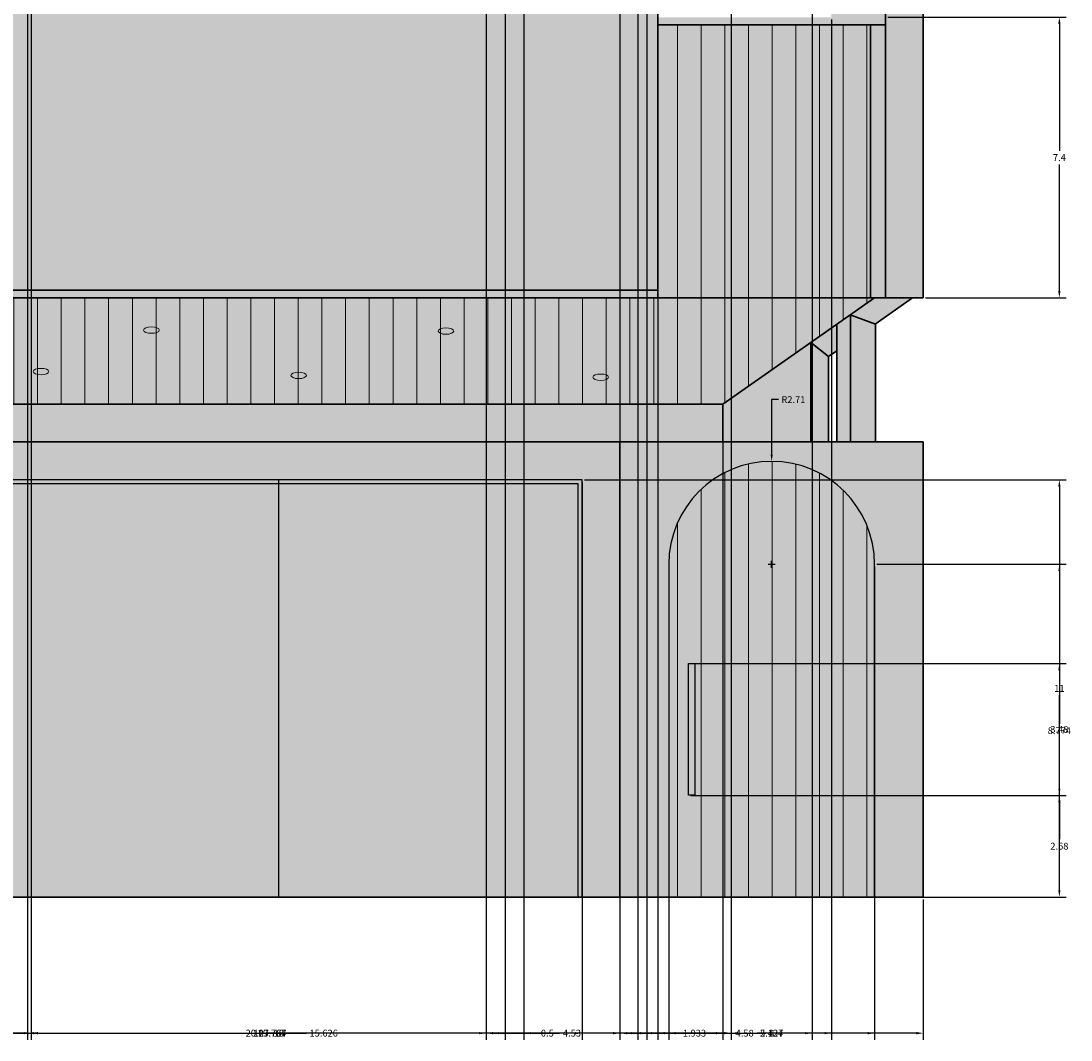
# Model space of a CAD drawing. Units: inches. Extents: x 18 to 59.8, y 2.7 to 81.2.
# Tile 2 of 9: x 32.1 to 59.8, y 2.7 to 29.5. Entities that reach past the tile are written whole.
import ezdxf

# ---------------------------------------------------------------- set-up
doc = ezdxf.new("R2010")
doc.units = ezdxf.units.IN
doc.header["$MEASUREMENT"] = 0
for name, color, linetype, lineweight in [('A-ANNO-DIMS', 2, 'Continuous', 18), ('A-DOOR', 3, 'Continuous', 25), ('A-ELEV', 7, 'Continuous', 35), ('A-ELEV-PATT', 8, 'Continuous', 13), ('E-LITE', 2, 'Continuous', 18)]:
    doc.layers.add(name, color=color, linetype=linetype, lineweight=lineweight)
doc.styles.get("Standard").update_dxf_attribs({"font": 'arial.ttf'})
doc.dimstyles.get("Standard").update_dxf_attribs({"dimtxt": 0.18, "dimasz": 0.18, "dimexe": 0.18, "dimexo": 0.0625, "dimgap": 0.09, "dimtad": 0, "dimtih": 1, "dimtoh": 1, "dimdec": 1, "dimzin": 0, "dimdsep": 46, "dimlunit": 3, "dimtxsty": 'Standard', "dimcen": 0.09, "dimadec": 0, "dimazin": 0, "dimtfac": 1, "dimtdec": 1, "dimtofl": 0, "dimtmove": 0, "dimatfit": 3, "dimfxl": 1, "dimtolj": 1, "dimtzin": 0, "dimarcsym": 0})

# ---------------------------------------------------------------- blocks, each defined once
blk = doc.blocks.new('LIGHT-SOFFIT-DOWN')
blk.add_ellipse((0.199, 0.085), major_axis=(0.207, 0), ratio=0.411448)
blk = doc.blocks.new('*D15')
at = {"layer": 'A-ANNO-DIMS', "color": 0, "lineweight": -2, "transparency": 16777216}
for p, q in [((54.922471, 29.640748), (59.629971, 29.640748)), ((59.449971, 29.460748), (59.449971, 26.120748)), ((59.449971, 22.420748), (59.449971, 25.760748)), ((55.922471, 22.240748), (59.629971, 22.240748))]:
    blk.add_line(p, q, dxfattribs=at)
at = {"layer": 'A-ANNO-DIMS', "color": 0, "transparency": 16777216}
for points in [[(59.419971, 29.460748), (59.479971, 29.460748), (59.449971, 29.640748)], [(59.419971, 22.420748), (59.479971, 22.420748), (59.449971, 22.240748)]]:
    blk.add_solid(points, dxfattribs=at)
at = {"layer": 'Defpoints', "color": 0, "transparency": 16777216}
for p in [(54.859971, 29.640748), (59.449971, 29.640748), (55.859971, 22.240748)]:
    blk.add_point(p, dxfattribs=at)
at = {"layer": 'A-ANNO-DIMS', "color": 0, "transparency": 16777216, "insert": (59.449971, 25.940748), "char_height": 0.18, "attachment_point": 5}
blk.add_mtext('\\A1;7.4', dxfattribs=at)
blk = doc.blocks.new('*D23')
at = {"layer": 'A-ANNO-DIMS', "color": 0, "lineweight": -2, "transparency": 16777216}
for p, q in [((48.86, 29.578), (48.86, 2.671)), ((53.44, 29.578), (53.44, 2.671)), ((49.04, 2.851), (50.822, 2.851)), ((53.26, 2.851), (51.478, 2.851))]:
    blk.add_line(p, q, dxfattribs=at)
at = {"layer": 'A-ANNO-DIMS', "color": 0, "transparency": 16777216}
for points in [[(49.04, 2.881), (49.04, 2.821), (48.86, 2.851)], [(53.26, 2.881), (53.26, 2.821), (53.44, 2.851)]]:
    blk.add_solid(points, dxfattribs=at)
at = {"layer": 'Defpoints', "color": 0, "transparency": 16777216}
for p in [(48.86, 29.641), (53.44, 29.641), (53.44, 2.851)]:
    blk.add_point(p, dxfattribs=at)
at = {"layer": 'A-ANNO-DIMS', "color": 0, "transparency": 16777216, "insert": (51.15, 2.851), "char_height": 0.18, "attachment_point": 5}
blk.add_mtext('\\A1;4.58', dxfattribs=at)
blk = doc.blocks.new('*D24')
at = {"layer": 'A-ANNO-DIMS', "color": 0, "lineweight": -2, "transparency": 16777216}
for p, q in [((48.86, 38.622), (48.86, 2.671)), ((50.793, 38.622), (50.793, 2.671)), ((49.04, 2.851), (49.441, 2.851)), ((50.613, 2.851), (50.212, 2.851))]:
    blk.add_line(p, q, dxfattribs=at)
at = {"layer": 'A-ANNO-DIMS', "color": 0, "transparency": 16777216}
for points in [[(49.04, 2.881), (49.04, 2.821), (48.86, 2.851)], [(50.613, 2.881), (50.613, 2.821), (50.793, 2.851)]]:
    blk.add_solid(points, dxfattribs=at)
at = {"layer": 'Defpoints', "color": 0, "transparency": 16777216}
for p in [(48.86, 38.685), (50.793, 38.685), (50.793, 2.851)]:
    blk.add_point(p, dxfattribs=at)
at = {"layer": 'A-ANNO-DIMS', "color": 0, "transparency": 16777216, "insert": (49.826, 2.851), "char_height": 0.18, "attachment_point": 5}
blk.add_mtext('\\A1;1.933', dxfattribs=at)
blk = doc.blocks.new('*D25')
at = {"layer": 'A-ANNO-DIMS', "color": 0, "lineweight": -2, "transparency": 16777216}
for p, q in [((50.793, 41.253), (50.793, 2.671)), ((52.927, 41.253), (52.927, 2.671)), ((50.973, 2.851), (51.465, 2.851)), ((52.747, 2.851), (52.255, 2.851))]:
    blk.add_line(p, q, dxfattribs=at)
at = {"layer": 'A-ANNO-DIMS', "color": 0, "transparency": 16777216}
for points in [[(50.973, 2.881), (50.973, 2.821), (50.793, 2.851)], [(52.747, 2.881), (52.747, 2.821), (52.927, 2.851)]]:
    blk.add_solid(points, dxfattribs=at)
at = {"layer": 'Defpoints', "color": 0, "transparency": 16777216}
for p in [(50.793, 41.316), (52.927, 41.316), (52.927, 2.851)]:
    blk.add_point(p, dxfattribs=at)
at = {"layer": 'A-ANNO-DIMS', "color": 0, "transparency": 16777216, "insert": (51.86, 2.851), "char_height": 0.18, "attachment_point": 5}
blk.add_mtext('\\A1;2.134', dxfattribs=at)
blk = doc.blocks.new('*D29')
at = {"layer": 'A-ANNO-DIMS', "color": 0, "lineweight": -2, "transparency": 16777216}
for p, q in [((29.86, 6.378), (29.86, 2.671)), ((47.86, 6.378), (47.86, 2.671)), ((30.04, 2.851), (38.649, 2.851)), ((47.68, 2.851), (39.071, 2.851))]:
    blk.add_line(p, q, dxfattribs=at)
at = {"layer": 'A-ANNO-DIMS', "color": 0, "transparency": 16777216}
for points in [[(30.04, 2.881), (30.04, 2.821), (29.86, 2.851)], [(47.68, 2.881), (47.68, 2.821), (47.86, 2.851)]]:
    blk.add_solid(points, dxfattribs=at)
at = {"layer": 'Defpoints', "color": 0, "transparency": 16777216}
for p in [(29.86, 6.441), (47.86, 6.441), (47.86, 2.851)]:
    blk.add_point(p, dxfattribs=at)
at = {"layer": 'A-ANNO-DIMS', "color": 0, "transparency": 16777216, "insert": (38.86, 2.851), "char_height": 0.18, "attachment_point": 5}
blk.add_mtext('\\A1;18', dxfattribs=at)
blk = doc.blocks.new('*D30')
at = {"layer": 'A-ANNO-DIMS', "color": 0, "lineweight": -2, "transparency": 16777216}
for p, q in [((47.86, 6.378), (47.86, 2.671)), ((55.86, 6.378), (55.86, 2.671)), ((48.04, 2.851), (51.711, 2.851)), ((55.68, 2.851), (52.009, 2.851))]:
    blk.add_line(p, q, dxfattribs=at)
at = {"layer": 'A-ANNO-DIMS', "color": 0, "transparency": 16777216}
for points in [[(48.04, 2.881), (48.04, 2.821), (47.86, 2.851)], [(55.68, 2.881), (55.68, 2.821), (55.86, 2.851)]]:
    blk.add_solid(points, dxfattribs=at)
at = {"layer": 'Defpoints', "color": 0, "transparency": 16777216}
for p in [(47.86, 6.441), (55.86, 6.441), (55.86, 2.851)]:
    blk.add_point(p, dxfattribs=at)
at = {"layer": 'A-ANNO-DIMS', "color": 0, "transparency": 16777216, "insert": (51.86, 2.851), "char_height": 0.18, "attachment_point": 5}
blk.add_mtext('\\A1;8', dxfattribs=at)
blk = doc.blocks.new('*D33')
at = {"layer": 'A-ANNO-DIMS', "color": 0, "lineweight": -2, "transparency": 16777216}
for p, q in [((49.148, 15.152), (49.148, 2.671)), ((54.576, 15.152), (54.576, 2.671)), ((49.328, 2.851), (51.468, 2.851)), ((54.396, 2.851), (52.256, 2.851))]:
    blk.add_line(p, q, dxfattribs=at)
at = {"layer": 'A-ANNO-DIMS', "color": 0, "transparency": 16777216}
for points in [[(49.328, 2.881), (49.328, 2.821), (49.148, 2.851)], [(54.396, 2.881), (54.396, 2.821), (54.576, 2.851)]]:
    blk.add_solid(points, dxfattribs=at)
at = {"layer": 'Defpoints', "color": 0, "transparency": 16777216}
for p in [(49.148, 15.215), (54.576, 15.215), (54.576, 2.851)]:
    blk.add_point(p, dxfattribs=at)
at = {"layer": 'A-ANNO-DIMS', "color": 0, "transparency": 16777216, "insert": (51.862, 2.851), "char_height": 0.18, "attachment_point": 5}
blk.add_mtext('\\A1;5.427', dxfattribs=at)
blk = doc.blocks.new('*D34')
at = {"layer": 'A-ANNO-DIMS', "color": 0, "lineweight": -2, "transparency": 16777216}
for p, q in [((30.86, 17.378), (30.86, 2.671)), ((46.86, 17.378), (46.86, 2.671)), ((31.04, 2.851), (38.65, 2.851)), ((46.68, 2.851), (39.07, 2.851))]:
    blk.add_line(p, q, dxfattribs=at)
at = {"layer": 'A-ANNO-DIMS', "color": 0, "transparency": 16777216}
for points in [[(31.04, 2.881), (31.04, 2.821), (30.86, 2.851)], [(46.68, 2.881), (46.68, 2.821), (46.86, 2.851)]]:
    blk.add_solid(points, dxfattribs=at)
at = {"layer": 'Defpoints', "color": 0, "transparency": 16777216}
for p in [(30.86, 17.441), (46.86, 17.441), (46.86, 2.851)]:
    blk.add_point(p, dxfattribs=at)
at = {"layer": 'A-ANNO-DIMS', "color": 0, "transparency": 16777216, "insert": (38.86, 2.851), "char_height": 0.18, "attachment_point": 5}
blk.add_mtext('\\A1;16', dxfattribs=at)
blk = doc.blocks.new('*D41')
at = {"layer": 'A-ANNO-DIMS', "color": 0, "lineweight": -2, "transparency": 16777216}
for p, q in [((54.638, 15.215), (59.63, 15.215)), ((59.45, 15.035), (59.45, 11.01)), ((59.45, 6.621), (59.45, 10.646)), ((54.638, 6.441), (59.63, 6.441))]:
    blk.add_line(p, q, dxfattribs=at)
at = {"layer": 'A-ANNO-DIMS', "color": 0, "transparency": 16777216}
for points in [[(59.42, 15.035), (59.48, 15.035), (59.45, 15.215)], [(59.42, 6.621), (59.48, 6.621), (59.45, 6.441)]]:
    blk.add_solid(points, dxfattribs=at)
at = {"layer": 'Defpoints', "color": 0, "transparency": 16777216}
for p in [(54.576, 15.215), (59.45, 15.215), (54.576, 6.441)]:
    blk.add_point(p, dxfattribs=at)
at = {"layer": 'A-ANNO-DIMS', "color": 0, "transparency": 16777216, "insert": (59.45, 10.828), "char_height": 0.18, "attachment_point": 5}
blk.add_mtext('\\A1;8.774', dxfattribs=at)
blk = doc.blocks.new('*D42')
at = {"layer": 'A-ANNO-DIMS', "color": 0, "lineweight": -2, "transparency": 16777216}
for p, q in [((46.922, 17.441), (59.63, 17.441)), ((59.45, 17.261), (59.45, 12.121)), ((59.45, 6.621), (59.45, 11.76)), ((46.922, 6.441), (59.63, 6.441))]:
    blk.add_line(p, q, dxfattribs=at)
at = {"layer": 'A-ANNO-DIMS', "color": 0, "transparency": 16777216}
for points in [[(59.42, 17.261), (59.48, 17.261), (59.45, 17.441)], [(59.42, 6.621), (59.48, 6.621), (59.45, 6.441)]]:
    blk.add_solid(points, dxfattribs=at)
at = {"layer": 'Defpoints', "color": 0, "transparency": 16777216}
for p in [(46.86, 17.441), (59.45, 17.441), (46.86, 6.441)]:
    blk.add_point(p, dxfattribs=at)
at = {"layer": 'A-ANNO-DIMS', "color": 0, "transparency": 16777216, "insert": (59.45, 11.941), "char_height": 0.18, "attachment_point": 5}
blk.add_mtext('\\A1;11', dxfattribs=at)
blk = doc.blocks.new('*D43')
at = {"layer": 'A-ANNO-DIMS', "color": 0, "lineweight": -2, "transparency": 16777216}
for p, q in [((49.728, 12.602), (59.63, 12.602)), ((59.45, 12.422), (59.45, 11.044)), ((59.45, 9.302), (59.45, 10.68)), ((49.728, 9.122), (59.63, 9.122))]:
    blk.add_line(p, q, dxfattribs=at)
at = {"layer": 'A-ANNO-DIMS', "color": 0, "transparency": 16777216}
for points in [[(59.42, 12.422), (59.48, 12.422), (59.45, 12.602)], [(59.42, 9.302), (59.48, 9.302), (59.45, 9.122)]]:
    blk.add_solid(points, dxfattribs=at)
at = {"layer": 'Defpoints', "color": 0, "transparency": 16777216}
for p in [(49.666, 12.602), (59.45, 12.602), (49.666, 9.122)]:
    blk.add_point(p, dxfattribs=at)
at = {"layer": 'A-ANNO-DIMS', "color": 0, "transparency": 16777216, "insert": (59.45, 10.862), "char_height": 0.18, "attachment_point": 5}
blk.add_mtext('\\A1;3.48', dxfattribs=at)
blk = doc.blocks.new('*D44')
at = {"layer": 'A-ANNO-DIMS', "color": 0, "lineweight": -2, "transparency": 16777216}
for p, q in [((49.728, 9.122), (59.63, 9.122)), ((59.45, 8.942), (59.45, 7.964)), ((59.45, 6.621), (59.45, 7.6)), ((49.211, 6.441), (59.63, 6.441))]:
    blk.add_line(p, q, dxfattribs=at)
at = {"layer": 'A-ANNO-DIMS', "color": 0, "transparency": 16777216}
for points in [[(59.42, 8.942), (59.48, 8.942), (59.45, 9.122)], [(59.42, 6.621), (59.48, 6.621), (59.45, 6.441)]]:
    blk.add_solid(points, dxfattribs=at)
at = {"layer": 'Defpoints', "color": 0, "transparency": 16777216}
for p in [(49.666, 9.122), (59.45, 9.122), (49.148, 6.441)]:
    blk.add_point(p, dxfattribs=at)
at = {"layer": 'A-ANNO-DIMS', "color": 0, "transparency": 16777216, "insert": (59.45, 7.782), "char_height": 0.18, "attachment_point": 5}
blk.add_mtext('\\A1;2.68', dxfattribs=at)
blk = doc.blocks.new('*D46')
at = {"layer": 'A-ANNO-DIMS', "color": 0, "lineweight": -2, "transparency": 16777216}
for p, q in [((26.811, 19.378), (26.811, 2.671)), ((50.578, 19.378), (50.578, 2.671)), ((26.991, 2.851), (38.229, 2.851)), ((50.398, 2.851), (39.159, 2.851))]:
    blk.add_line(p, q, dxfattribs=at)
at = {"layer": 'A-ANNO-DIMS', "color": 0, "transparency": 16777216}
for points in [[(26.991, 2.881), (26.991, 2.821), (26.811, 2.851)], [(50.398, 2.881), (50.398, 2.821), (50.578, 2.851)]]:
    blk.add_solid(points, dxfattribs=at)
at = {"layer": 'Defpoints', "color": 0, "transparency": 16777216}
for p in [(26.811, 19.441), (50.578, 19.441), (50.578, 2.851)]:
    blk.add_point(p, dxfattribs=at)
at = {"layer": 'A-ANNO-DIMS', "color": 0, "transparency": 16777216, "insert": (38.694, 2.851), "char_height": 0.18, "attachment_point": 5}
blk.add_mtext('\\A1;23.767', dxfattribs=at)
blk = doc.blocks.new('*D54')
at = {"layer": 'A-ANNO-DIMS', "color": 0, "lineweight": -2, "transparency": 16777216}
for p, q in [((28.258, 33.771), (28.258, 2.671)), ((48.33, 33.352), (48.33, 2.671)), ((28.438, 2.851), (37.899, 2.851)), ((48.15, 2.851), (38.689, 2.851))]:
    blk.add_line(p, q, dxfattribs=at)
at = {"layer": 'A-ANNO-DIMS', "color": 0, "transparency": 16777216}
for points in [[(28.438, 2.881), (28.438, 2.821), (28.258, 2.851)], [(48.15, 2.881), (48.15, 2.821), (48.33, 2.851)]]:
    blk.add_solid(points, dxfattribs=at)
at = {"layer": 'Defpoints', "color": 0, "transparency": 16777216}
for p in [(28.258, 33.834), (48.33, 33.414), (48.33, 2.851)]:
    blk.add_point(p, dxfattribs=at)
at = {"layer": 'A-ANNO-DIMS', "color": 0, "transparency": 16777216, "insert": (38.294, 2.851), "char_height": 0.18, "attachment_point": 5}
blk.add_mtext('\\A1;20.07', dxfattribs=at)
blk = doc.blocks.new('*D55')
at = {"layer": 'A-ANNO-DIMS', "color": 0, "lineweight": -2, "transparency": 16777216}
for p, q in [((44.83, 33.671), (44.83, 2.671)), ((45.33, 33.671), (45.33, 2.671)), ((44.65, 2.851), (44.47, 2.851)), ((45.51, 2.851), (45.69, 2.851))]:
    blk.add_line(p, q, dxfattribs=at)
at = {"layer": 'A-ANNO-DIMS', "color": 0, "transparency": 16777216}
for points in [[(44.65, 2.881), (44.65, 2.821), (44.83, 2.851)], [(45.51, 2.881), (45.51, 2.821), (45.33, 2.851)]]:
    blk.add_solid(points, dxfattribs=at)
at = {"layer": 'Defpoints', "color": 0, "transparency": 16777216}
for p in [(44.83, 33.734), (45.33, 33.734), (45.33, 2.851)]:
    blk.add_point(p, dxfattribs=at)
at = {"layer": 'A-ANNO-DIMS', "color": 0, "transparency": 16777216, "insert": (45.945, 2.851), "char_height": 0.18, "attachment_point": 5}
blk.add_mtext('\\A1;0.5', dxfattribs=at)
blk = doc.blocks.new('*D56')
at = {"layer": 'A-ANNO-DIMS', "color": 0, "lineweight": -2, "transparency": 16777216}
for p, q in [((30.406, 31.378), (30.406, 2.671)), ((32.33, 31.378), (32.33, 2.671)), ((30.586, 2.851), (30.983, 2.851)), ((32.15, 2.851), (31.753, 2.851))]:
    blk.add_line(p, q, dxfattribs=at)
at = {"layer": 'A-ANNO-DIMS', "color": 0, "transparency": 16777216}
for points in [[(30.586, 2.881), (30.586, 2.821), (30.406, 2.851)], [(32.15, 2.881), (32.15, 2.821), (32.33, 2.851)]]:
    blk.add_solid(points, dxfattribs=at)
at = {"layer": 'Defpoints', "color": 0, "transparency": 16777216}
for p in [(30.406, 31.441), (32.33, 31.441), (32.33, 2.851)]:
    blk.add_point(p, dxfattribs=at)
at = {"layer": 'A-ANNO-DIMS', "color": 0, "transparency": 16777216, "insert": (31.368, 2.851), "char_height": 0.18, "attachment_point": 5}
blk.add_mtext('\\A1;1.924', dxfattribs=at)
blk = doc.blocks.new('*D57')
at = {"layer": 'A-ANNO-DIMS', "color": 0, "lineweight": -2, "transparency": 16777216}
for p, q in [((32.33, 31.378), (32.33, 2.671)), ((44.33, 31.378), (44.33, 2.671)), ((32.51, 2.851), (38.121, 2.851)), ((44.15, 2.851), (38.54, 2.851))]:
    blk.add_line(p, q, dxfattribs=at)
at = {"layer": 'A-ANNO-DIMS', "color": 0, "transparency": 16777216}
for points in [[(32.51, 2.881), (32.51, 2.821), (32.33, 2.851)], [(44.15, 2.881), (44.15, 2.821), (44.33, 2.851)]]:
    blk.add_solid(points, dxfattribs=at)
at = {"layer": 'Defpoints', "color": 0, "transparency": 16777216}
for p in [(32.33, 31.441), (44.33, 31.441), (44.33, 2.851)]:
    blk.add_point(p, dxfattribs=at)
at = {"layer": 'A-ANNO-DIMS', "color": 0, "transparency": 16777216, "insert": (38.33, 2.851), "char_height": 0.18, "attachment_point": 5}
blk.add_mtext('\\A1;12', dxfattribs=at)
blk = doc.blocks.new('*D58')
at = {"layer": 'A-ANNO-DIMS', "color": 0, "lineweight": -2, "transparency": 16777216}
for p, q in [((48.86, 38.622), (48.86, 2.671)), ((44.33, 31.378), (44.33, 2.671)), ((44.51, 2.851), (46.268, 2.851)), ((48.68, 2.851), (46.923, 2.851))]:
    blk.add_line(p, q, dxfattribs=at)
at = {"layer": 'A-ANNO-DIMS', "color": 0, "transparency": 16777216}
for points in [[(44.51, 2.881), (44.51, 2.821), (44.33, 2.851)], [(48.68, 2.881), (48.68, 2.821), (48.86, 2.851)]]:
    blk.add_solid(points, dxfattribs=at)
at = {"layer": 'Defpoints', "color": 0, "transparency": 16777216}
for p in [(48.86, 38.685), (44.33, 31.441), (48.86, 2.851)]:
    blk.add_point(p, dxfattribs=at)
at = {"layer": 'A-ANNO-DIMS', "color": 0, "transparency": 16777216, "insert": (46.595, 2.851), "char_height": 0.18, "attachment_point": 5}
blk.add_mtext('\\A1;4.53', dxfattribs=at)
blk = doc.blocks.new('*D61')
at = {"layer": 'A-ANNO-DIMS', "color": 0, "lineweight": -2, "transparency": 16777216}
for p, q in [((32.234, 49.378), (32.234, 2.671)), ((47.86, 49.378), (47.86, 2.671)), ((32.414, 2.851), (39.592, 2.851)), ((47.68, 2.851), (40.502, 2.851))]:
    blk.add_line(p, q, dxfattribs=at)
at = {"layer": 'A-ANNO-DIMS', "color": 0, "transparency": 16777216}
for points in [[(32.414, 2.881), (32.414, 2.821), (32.234, 2.851)], [(47.68, 2.881), (47.68, 2.821), (47.86, 2.851)]]:
    blk.add_solid(points, dxfattribs=at)
at = {"layer": 'Defpoints', "color": 0, "transparency": 16777216}
for p in [(32.234, 49.441), (47.86, 49.441), (47.86, 2.851)]:
    blk.add_point(p, dxfattribs=at)
at = {"layer": 'A-ANNO-DIMS', "color": 0, "transparency": 16777216, "insert": (40.047, 2.851), "char_height": 0.18, "attachment_point": 5}
blk.add_mtext('\\A1;15.626', dxfattribs=at)
blk = doc.blocks.new('*D66')
at = {"layer": 'A-ANNO-DIMS', "color": 0, "lineweight": -2, "transparency": 16777216}
for p, q in [((28.804, 51.378), (28.804, 2.671)), ((48.567, 51.179), (48.567, 2.671)), ((28.984, 2.851), (38.231, 2.851)), ((48.387, 2.851), (39.14, 2.851))]:
    blk.add_line(p, q, dxfattribs=at)
at = {"layer": 'A-ANNO-DIMS', "color": 0, "transparency": 16777216}
for points in [[(28.984, 2.881), (28.984, 2.821), (28.804, 2.851)], [(48.387, 2.881), (48.387, 2.821), (48.567, 2.851)]]:
    blk.add_solid(points, dxfattribs=at)
at = {"layer": 'Defpoints', "color": 0, "transparency": 16777216}
for p in [(28.804, 51.441), (48.567, 51.242), (48.567, 2.851)]:
    blk.add_point(p, dxfattribs=at)
at = {"layer": 'A-ANNO-DIMS', "color": 0, "transparency": 16777216, "insert": (38.685, 2.851), "char_height": 0.18, "attachment_point": 5}
blk.add_mtext('\\A1;19.764', dxfattribs=at)
blk = doc.blocks.new('*D68')
at = {"layer": 'A-ANNO-DIMS', "color": 0, "lineweight": -2, "transparency": 16777216}
for p, q in [((52.042, 19.557), (51.862, 19.557)), ((51.862, 19.557), (51.862, 18.109)), ((51.862, 15.125), (51.862, 15.305)), ((51.772, 15.215), (51.952, 15.215))]:
    blk.add_line(p, q, dxfattribs=at)
at = {"layer": 'A-ANNO-DIMS', "color": 0, "transparency": 16777216}
blk.add_solid([(51.832, 18.109), (51.892, 18.109), (51.862, 17.929)], dxfattribs=at)
at = {"layer": 'Defpoints', "color": 0, "transparency": 16777216}
for p in [(51.862, 17.929), (51.862, 15.215)]:
    blk.add_point(p, dxfattribs=at)
at = {"layer": 'A-ANNO-DIMS', "color": 0, "transparency": 16777216, "insert": (52.435, 19.557), "char_height": 0.18, "attachment_point": 5}
blk.add_mtext('\\A1;R2.71', dxfattribs=at)

msp = doc.modelspace()

# ---------------------------------------------------------------- hatches: boundary and pattern name
at = {"layer": 'A-ELEV-PATT'}
h = msp.add_hatch(color=256, dxfattribs=at)
h.set_gradient(color1=(255, 255, 255), color2=(199, 200, 202))
h.paths.add_polyline_path([(38.86, 75.4521, 0.4125527), (36.86, 77.4407), (21.86, 77.4407), (21.86, 22.4407), (22.86, 22.4407), (48.86, 22.4407), (48.86, 30.9234, 0.4074473), (48.3302, 31.4407), (30.4061, 31.4407, -0.7603989), (34.0116, 44.4407), (47.86, 44.4407, -0.4142136), (48.86, 43.4407), (48.86, 48.4407, 0.4142136), (47.86, 49.4407), (32.2338, 49.4407, -0.2243142), (27.8411, 52.8427, -0.8480129), (38.86, 61.4407)])
h.paths.add_polyline_path([(55.86, 77.4407), (54.86, 77.4407), (54.86, 22.2407), (55.86, 22.2407)])
h.paths.add_polyline_path([(54.86, 51.5407), (53.4401, 51.5407), (53.4401, 29.6407), (54.86, 29.6407)])
h.paths.add_polyline_path([(54.86, 61.4407), (53.4401, 57.4407), (53.4401, 51.6407), (54.86, 51.6407)])
h.paths.add_polyline_path([(54.86, 29.4407), (54.471, 29.4407), (54.471, 22.2407), (54.86, 22.2407)])
h.paths.add_polyline_path([(55.5745, 22.2407), (54.86, 22.2407), (54.5745, 22.2407), (53.9347, 21.7925), (54.5877, 21.5495)])
h.paths.add_polyline_path([(54.5991, 21.5452), (53.9443, 21.789), (53.9443, 18.4407), (54.5991, 18.4407)])
h.paths.add_polyline_path([(53.9443, 21.789), (53.9347, 21.7925), (53.5816, 21.5452), (53.5816, 18.4407), (53.9443, 18.4407)])
h.paths.add_polyline_path([(53.3648, 20.6928), (52.8956, 21.0646), (52.8956, 18.4407), (53.3648, 18.4407)])
h.paths.add_polyline_path([(52.8956, 21.0646), (50.5775, 19.4407), (50.5775, 18.4407), (52.8956, 18.4407)])
h.paths.add_polyline_path([(53.5816, 21.5452), (52.8956, 21.0646), (53.3648, 20.6928), (53.5816, 20.8447)])
h.paths.add_polyline_path([(26.8109, 19.4407), (24.9672, 20.8407), (24.9672, 18.4407), (26.8109, 18.4407)])
h.paths.add_polyline_path([(24.9672, 20.8407), (24.4165, 20.8427), (24.4165, 18.4407), (24.9672, 18.4407)])
h.paths.add_polyline_path([(24.4165, 20.8427), (24.4165, 21.2589), (24.0588, 21.5305), (24.0301, 21.5183), (24.0301, 18.4407), (24.4165, 18.4407)])
h.paths.add_polyline_path([(24.0301, 21.5183), (23.4165, 21.2589), (23.4165, 18.4407), (24.0301, 18.4407)])
h.paths.add_polyline_path([(24.0301, 21.5183), (24.0588, 21.5305), (23.1234, 22.2407), (22.1234, 22.2407), (23.4165, 21.2589)])
h.paths.add_polyline_path([(24.4165, 21.2589), (24.4165, 20.8427), (24.9672, 20.8407)])
h.paths.add_polyline_path([(47.86, 18.4407), (29.86, 18.4407), (29.86, 6.4407), (30.86, 6.4407), (30.86, 17.4407), (38.86, 17.4407), (46.86, 17.4407), (46.86, 6.4407), (47.86, 6.4407)])
h.paths.add_polyline_path([(54.5756, 15.215), (54.5756, 6.4407), (55.86, 6.4407), (55.86, 18.4407), (47.86, 18.4407), (47.86, 6.4407), (49.1482, 6.4407), (49.1482, 15.215, -1)])
h = msp.add_hatch(color=256, dxfattribs=at)
h.paths.add_polyline_path([(27.8411, 52.8427, -0.7443789), (36.86, 61.4407), (38.86, 61.4407, 0.8480129)])
h.paths.add_polyline_path([(47.86, 44.4407), (34.0116, 44.4407, 0.7603989), (30.4061, 31.4407, -0.7376246), (34.0116, 43.4407), (47.86, 43.4407, -0.4142136), (48.86, 42.4407), (48.86, 43.4407, 0.4142136)])
h.paths.add_polyline_path([(54.5756, 15.215), (54.5756, 6.4407), (55.86, 6.4407), (55.86, 18.4407), (47.86, 18.4407), (47.86, 6.4407), (49.1482, 6.4407), (49.1482, 15.215, -1)])
h.paths.add_polyline_path([(47.86, 18.4407), (29.86, 18.4407), (29.86, 6.4407), (30.86, 6.4407), (30.86, 17.4407), (38.86, 17.4407), (46.86, 17.4407), (46.86, 6.4407), (47.86, 6.4407)])
h.paths.add_polyline_path([(55.86, 77.4407), (54.86, 77.4407), (54.86, 22.2407), (55.86, 22.2407)])
h = msp.add_hatch(color=256, dxfattribs=at)
h.dxf.hatch_style = 1
h.paths.add_polyline_path([(54.86, 69.4407), (38.86, 69.4407), (38.86, 61.4407), (54.86, 61.4407)])
h.paths.add_polyline_path([(54.86, 61.4407), (38.86, 61.4407), (36.86, 61.4407, 0.443414), (27.6986, 58.4407), (48.86, 58.4407), (48.86, 57.4407), (53.4401, 57.4407)])
h.paths.add_polyline_path([(37.4994, 59.9399), (37.4994, 59.8198, -2.4106499), (37.1187, 59.8198), (37.1187, 59.9399)], flags=16)
h.paths.add_polyline_path([(42.6125, 59.8012), (42.6125, 59.9213), (42.9933, 59.9213), (42.9933, 59.8012, -2.4106499)], flags=16)
h.paths.add_polyline_path([(49.5965, 59.971), (49.5965, 60.091), (49.9773, 60.091), (49.9773, 59.971, -2.4106499)], flags=16)
h.paths.add_polyline_path([(44.4671, 57.0407), (32.6671, 57.0407), (32.6671, 56.0407), (44.4671, 56.0407)])
h.paths.add_polyline_path([(47.86, 43.4407), (46.86, 43.4407), (34.0116, 43.4407, 0.2012983), (29.3481, 41.4407), (47.86, 41.4407, 1)])
h.paths.add_polyline_path([(36.5542, 42.5145), (36.5542, 42.6346), (36.9349, 42.6346), (36.9349, 42.5145, -2.4106499)], flags=16)
h.paths.add_polyline_path([(42.939, 42.5402), (42.939, 42.6603), (43.3198, 42.6603), (43.3198, 42.5402, -2.4106499)], flags=16)
h.paths.add_polyline_path([(54.471, 29.4407), (48.86, 29.4407), (48.86, 22.2407), (54.471, 22.2407)])
h.paths.add_polyline_path([(54.5745, 22.2407), (23.1234, 22.2407), (26.8109, 19.4407), (50.5775, 19.4407)])
h.paths.add_polyline_path([(54.5756, 15.215, 1), (49.1482, 15.215), (49.1482, 6.4407), (54.5756, 6.4407)])
h.paths.add_polyline_path([(49.8323, 12.602), (49.8323, 9.1225), (49.6657, 9.1225), (49.6657, 12.602)], flags=16)
h = msp.add_hatch(dxfattribs=at)
h.set_pattern_fill('ANSI31', color=256, scale=5, angle=45, style=0)
h.paths.add_polyline_path([(54.86, 69.4407), (38.86, 69.4407), (38.86, 61.4407), (54.86, 61.4407)])
h.paths.add_polyline_path([(54.86, 61.4407), (38.86, 61.4407), (36.86, 61.4407, 0.443414), (27.6986, 58.4407), (48.86, 58.4407), (48.86, 57.4407), (53.4401, 57.4407)])
h.paths.add_polyline_path([(37.1661, 59.8577), (37.1187, 59.8577), (37.1187, 59.9399), (37.4994, 59.9399), (37.4994, 59.8577), (37.452, 59.8577, -3.476462)], flags=16)
h.paths.add_polyline_path([(42.66, 59.8391), (42.6125, 59.8391), (42.6125, 59.9213), (42.9933, 59.9213), (42.9933, 59.8391), (42.9458, 59.8391, -3.476462)], flags=16)
h.paths.add_polyline_path([(49.644, 60.0088), (49.5965, 60.0088), (49.5965, 60.091), (49.9773, 60.091), (49.9773, 60.0088), (49.9298, 60.0088, -3.476462)], flags=16)
h.paths.add_polyline_path([(44.4671, 57.0407), (32.6671, 57.0407), (32.6671, 56.0407), (44.4671, 56.0407)])
h.paths.add_polyline_path([(47.86, 43.4407), (46.86, 43.4407), (34.0116, 43.4407, 0.2012983), (29.3481, 41.4407), (47.86, 41.4407, 1)])
h.paths.add_polyline_path([(36.6016, 42.5524), (36.5542, 42.5524), (36.5542, 42.6346), (36.9349, 42.6346), (36.9349, 42.5524), (36.8875, 42.5524, -3.476462)], flags=16)
h.paths.add_polyline_path([(42.9865, 42.578), (42.939, 42.578), (42.939, 42.6603), (43.3198, 42.6603), (43.3198, 42.578), (43.2723, 42.578, -3.476462)], flags=16)
h.paths.add_polyline_path([(54.471, 29.4407), (48.86, 29.4407), (48.86, 22.2407), (54.471, 22.2407)])
h.paths.add_polyline_path([(54.5745, 22.2407), (23.1234, 22.2407), (26.8109, 19.4407), (50.5775, 19.4407)])
h.paths.add_polyline_path([(54.5756, 15.215, 1), (49.1482, 15.215), (49.1482, 6.4407), (54.5756, 6.4407)])
h.paths.add_polyline_path([(49.8323, 9.1225), (49.6657, 9.1225), (49.6657, 12.602), (49.8323, 12.602)], flags=16)
h = msp.add_hatch(color=256, dxfattribs=at)
h.paths.add_polyline_path([(36.8875, 42.5524), (36.6016, 42.5524, 3.476462)])
h.paths.add_polyline_path([(43.2723, 42.578), (42.9865, 42.578, 3.476462)])
h.paths.add_polyline_path([(37.452, 59.8577), (37.1661, 59.8577, 3.476462)])
h.paths.add_polyline_path([(42.9458, 59.8391), (42.66, 59.8391, 3.476462)])
h.paths.add_polyline_path([(49.9298, 60.0088), (49.644, 60.0088, 3.476462)])
edge = h.paths.add_edge_path()
edge.add_ellipse((29.0313, 21.3107), major_axis=(-0.2068, 0), ratio=0.411448, start_angle=0, end_angle=360)
edge = h.paths.add_edge_path()
edge.add_ellipse((32.5919, 20.2963), major_axis=(-0.2068, 0), ratio=0.411448, start_angle=0, end_angle=360)
edge = h.paths.add_edge_path()
edge.add_ellipse((35.5044, 21.3908), major_axis=(-0.2068, 0), ratio=0.411448, start_angle=0, end_angle=360)
edge = h.paths.add_edge_path()
edge.add_ellipse((39.3877, 20.1968), major_axis=(-0.2068, 0), ratio=0.411448, start_angle=0, end_angle=360)
edge = h.paths.add_edge_path()
edge.add_ellipse((43.271, 21.3659), major_axis=(-0.2068, 0), ratio=0.411448, start_angle=0, end_angle=360)
edge = h.paths.add_edge_path()
edge.add_ellipse((47.3535, 20.1471), major_axis=(-0.2068, 0), ratio=0.411448, start_angle=0, end_angle=360)
h = msp.add_hatch(color=256, dxfattribs=at)
h.paths.add_polyline_path([(38.86, 17.4407), (30.86, 17.4407), (30.86, 6.4407), (30.96, 6.4407), (30.96, 17.3407), (38.86, 17.3407)])
h.paths.add_polyline_path([(46.86, 17.4407), (38.86, 17.4407), (38.86, 17.3407), (46.76, 17.3407), (46.76, 6.4407), (46.86, 6.4407)])
h.paths.add_polyline_path([(49.8323, 12.602), (49.6657, 12.602), (49.6657, 9.1225), (49.8323, 9.1225)])
h.paths.add_polyline_path([(48.86, 22.4407), (21.86, 22.4407), (21.86, 22.2407), (48.86, 22.2407)])
h.paths.add_polyline_path([(54.86, 29.6407), (48.86, 29.6407), (48.86, 29.4407), (54.86, 29.4407)])
edge = h.paths.add_edge_path()
edge.add_spline(control_points=[(48.3302, 33.5345), (48.1229, 33.671), (47.9155, 33.8074), (47.6839, 33.8336)], knot_values=[0, 0, 0, 0, 0.7121901, 0.7121901, 0.7121901, 0.7121901], degree=3, periodic=0)
edge.add_line((47.6839, 33.8336), (28.2583, 33.8336))
edge.add_arc((34.0631, 36.8836), 6.5573, 207.71831, 208.7099)
edge.add_line((28.3119, 33.7336), (47.6238, 33.7336))
edge.add_spline(control_points=[(47.6238, 33.7336), (47.6461, 33.7341), (47.6685, 33.7345), (47.6905, 33.7336)], knot_values=[0, 0, 0, 0, 0.0667446, 0.0667446, 0.0667446, 0.0667446], degree=3, periodic=0)
edge.add_spline(control_points=[(47.6905, 33.7336), (47.7384, 33.7318), (47.7849, 33.7239), (47.8302, 33.7113)], knot_values=[0.570104, 0.570104, 0.570104, 0.570104, 0.7151116, 0.7151116, 0.7151116, 0.7151116], degree=3, periodic=0)
edge.add_spline(control_points=[(47.8302, 33.7113), (48.0085, 33.6616), (48.1694, 33.5378), (48.3302, 33.4141)], knot_values=[0, 0, 0, 0, 0.570104, 0.570104, 0.570104, 0.570104], degree=3, periodic=0)
edge.add_line((48.3302, 33.4141), (48.3302, 33.5345))
h = msp.add_hatch(color=256, dxfattribs=at)
h.paths.add_polyline_path([(38.86, 17.3407), (30.96, 17.3407), (30.96, 6.4407), (38.86, 6.4407)])
h.paths.add_polyline_path([(46.76, 17.3407), (38.86, 17.3407), (38.86, 6.4407), (46.76, 6.4407)])
h.paths.add_polyline_path([(50.5775, 19.4407), (26.8109, 19.4407), (26.8109, 18.4407), (50.5775, 18.4407)])

# ---------------------------------------------------------------- linework, layer by layer
at = {"layer": 'A-DOOR'}
for p, q in [((38.86, 6.4407), (38.86, 17.4407)), ((49.1482, 15.215), (49.1482, 6.4407)), ((54.5756, 6.4407), (54.5756, 15.215)), ((49.1482, 6.4407), (54.5756, 6.4407))]:
    msp.add_line(p, q, dxfattribs=at)
for points in [[(46.86, 6.4407), (46.86, 17.4407), (38.86, 17.4407), (30.86, 17.4407), (30.86, 6.4407)], [(46.76, 6.4407), (46.76, 17.3407), (38.86, 17.3407), (30.96, 17.3407), (30.96, 6.4407)]]:
    msp.add_lwpolyline(points, dxfattribs=at)
msp.add_lwpolyline([(49.6657, 12.602), (49.8323, 12.602), (49.8323, 9.1225), (49.6657, 9.1225)], close=True, dxfattribs=at)
msp.add_arc((51.8619, 15.215), 2.7137, 0, 180, dxfattribs=at)
at = {"layer": 'A-ELEV'}
for p, q in [((54.86, 22.2407), (54.86, 77.4407)), ((55.86, 77.4407), (55.86, 22.2407)), ((48.86, 22.2407), (48.86, 38.6846)), ((54.86, 29.4407), (48.86, 29.4407)), ((54.471, 22.2407), (54.471, 29.4407)), ((21.86, 22.4407), (48.86, 22.4407)), ((21.86, 22.2407), (55.86, 22.2407)), ((54.5745, 22.2407), (50.5775, 19.4407)), ((55.5745, 22.2407), (54.5877, 21.5495)), ((53.9347, 21.7925), (54.5991, 21.5452)), ((53.9443, 21.789), (53.9443, 18.4407)), ((53.5816, 21.5452), (53.5816, 18.4407)), ((54.5991, 21.5575), (54.5991, 18.4407)), ((52.8956, 18.4407), (52.8956, 21.0646)), ((52.8956, 21.0646), (53.3648, 20.6928)), ((53.5816, 20.8447), (53.3648, 20.6928)), ((53.3648, 20.6928), (53.3648, 18.4407)), ((26.8109, 19.4407), (50.5775, 19.4407)), ((50.5775, 19.4407), (50.5775, 18.4407)), ((21.86, 18.4407), (55.86, 18.4407)), ((47.86, 6.4407), (47.86, 18.4407)), ((47.86, 18.4407), (47.86, 6.4407)), ((55.86, 6.4407), (55.86, 18.4407)), ((29.86, 6.4407), (47.86, 6.4407)), ((47.86, 6.4407), (55.86, 6.4407))]:
    msp.add_line(p, q, dxfattribs=at)

# ---------------------------------------------------------------- block references
at = {"layer": 'E-LITE', "rotation": 180}
for p in [(35.7032, 21.4755), (43.4699, 21.4506), (32.7907, 20.3811), (39.5865, 20.2816), (47.5523, 20.2318)]:
    msp.add_blockref('LIGHT-SOFFIT-DOWN', p, dxfattribs=at)

# ---------------------------------------------------------------- dimensions: what is measured, and where the dimension line sits
at = {"layer": 'A-ANNO-DIMS'}
for base, p1, p2, override, picture, middle in [((48.5671, 2.8507), (28.8035, 51.4407), (48.5671, 51.2416), {"dimdec": 3, "dimlfac": 1, "dimrnd": 0, "dimzin": 0, "dimdsep": 46, "dimlunit": 2}, '*D66', (38.6853, 2.8507)), ((47.86, 2.8507), (32.2338, 49.4407), (47.86, 49.4407), {"dimdec": 3, "dimlfac": 1, "dimrnd": 0, "dimzin": 0, "dimdsep": 46, "dimlunit": 2}, '*D61', (40.0469, 2.8507)), ((52.927, 2.8507), (50.793, 41.316), (52.927, 41.316), {"dimdec": 3, "dimlfac": 1, "dimrnd": 0, "dimzin": 0, "dimdsep": 46, "dimlunit": 2}, '*D25', (51.86, 2.8507)), ((48.86, 2.8507), (44.3302, 31.4407), (48.86, 38.6846), {"dimdec": 2, "dimlfac": 1, "dimrnd": 0, "dimzin": 0, "dimdsep": 46, "dimlunit": 2}, '*D58', (46.5951, 2.8507)), ((50.793, 2.8507), (48.86, 38.6846), (50.793, 38.6846), {"dimdec": 3, "dimlfac": 1, "dimrnd": 0, "dimzin": 0, "dimdsep": 46, "dimlunit": 2}, '*D24', (49.8265, 2.8507)), ((48.3302, 2.8507), (28.2583, 33.8336), (48.3302, 33.4141), {"dimdec": 2, "dimlfac": 1, "dimrnd": 0, "dimzin": 0, "dimdsep": 46, "dimlunit": 2}, '*D54', (38.2942, 2.8507)), ((45.3302, 2.8507), (44.8302, 33.7336), (45.3302, 33.7336), {"dimdec": 1, "dimlfac": 1, "dimrnd": 0, "dimzin": 0, "dimdsep": 46, "dimlunit": 2}, '*D55', (45.9448, 2.8507)), ((32.3302, 2.8507), (30.4061, 31.4407), (32.3302, 31.4407), {"dimdec": 3, "dimlfac": 1, "dimrnd": 0, "dimzin": 0, "dimdsep": 46, "dimlunit": 2}, '*D56', (31.3682, 2.8507)), ((44.3302, 2.8507), (32.3302, 31.4407), (44.3302, 31.4407), {"dimdec": 0, "dimlfac": 1, "dimrnd": 0, "dimzin": 0, "dimdsep": 46, "dimlunit": 2}, '*D57', (38.3302, 2.8507)), ((53.4401, 2.8507), (48.86, 29.6407), (53.4401, 29.6407), {"dimdec": 2, "dimlfac": 1, "dimrnd": 0, "dimzin": 0, "dimdsep": 46, "dimlunit": 2}, '*D23', (51.15, 2.8507)), ((50.5775, 2.8507), (26.8109, 19.4407), (50.5775, 19.4407), {"dimdec": 3, "dimlfac": 1, "dimrnd": 0, "dimzin": 0, "dimdsep": 46, "dimlunit": 2}, '*D46', (38.6942, 2.8507)), ((46.86, 2.8507), (30.86, 17.4407), (46.86, 17.4407), {"dimdec": 0, "dimlfac": 1, "dimrnd": 0, "dimzin": 0, "dimdsep": 46, "dimlunit": 2}, '*D34', (38.86, 2.8507)), ((54.5756, 2.8507), (49.1482, 15.215), (54.5756, 15.215), {"dimdec": 3, "dimlfac": 1, "dimrnd": 0, "dimzin": 0, "dimdsep": 46, "dimlunit": 2}, '*D33', (51.8619, 2.8507)), ((47.86, 2.8507), (29.86, 6.4407), (47.86, 6.4407), {"dimdec": 0, "dimlfac": 1, "dimrnd": 0, "dimzin": 0, "dimdsep": 46, "dimlunit": 2}, '*D29', (38.86, 2.8507)), ((55.86, 2.8507), (47.86, 6.4407), (55.86, 6.4407), {"dimdec": 0, "dimlfac": 1, "dimrnd": 0, "dimzin": 0, "dimdsep": 46, "dimlunit": 2}, '*D30', (51.86, 2.8507))]:
    dim = msp.add_linear_dim(base=base, p1=p1, p2=p2, dimstyle='Standard', override=override, dxfattribs=at)
    dim.commit()
    dim.dimension.update_dxf_attribs({"geometry": picture, "text_midpoint": middle})
for base, p1, p2, override, picture, middle in [((59.45, 29.6407), (55.86, 22.2407), (54.86, 29.6407), {"dimdec": 1, "dimlfac": 1, "dimrnd": 0, "dimzin": 0, "dimdsep": 46, "dimlunit": 2}, '*D15', (59.45, 25.9407)), ((59.45, 17.4407), (46.86, 6.4407), (46.86, 17.4407), {"dimdec": 0, "dimlfac": 1, "dimrnd": 0, "dimzin": 0, "dimdsep": 46, "dimlunit": 2}, '*D42', (59.45, 11.9407)), ((59.45, 15.215), (54.5756, 6.4407), (54.5756, 15.215), {"dimdec": 3, "dimlfac": 1, "dimrnd": 0, "dimzin": 0, "dimdsep": 46, "dimlunit": 2}, '*D41', (59.45, 10.8279)), ((59.45, 12.602), (49.6657, 9.1225), (49.6657, 12.602), {"dimdec": 2, "dimlfac": 1, "dimrnd": 0, "dimzin": 0, "dimdsep": 46, "dimlunit": 2}, '*D43', (59.45, 10.8622)), ((59.45, 9.1225), (49.1482, 6.4407), (49.6657, 9.1225), {"dimdec": 2, "dimlfac": 1, "dimrnd": 0, "dimzin": 0, "dimdsep": 46, "dimlunit": 2}, '*D44', (59.45, 7.7816))]:
    dim = msp.add_linear_dim(base=base, p1=p1, p2=p2, angle=90, dimstyle='Standard', override=override, dxfattribs=at)
    dim.commit()
    dim.dimension.update_dxf_attribs({"geometry": picture, "text_midpoint": middle})
dim = msp.add_radius_dim(center=(51.8619, 15.215), mpoint=(51.862, 17.9287), dimstyle='Standard', override={"dimdec": 2, "dimlfac": 1, "dimrnd": 0, "dimzin": 0, "dimdsep": 46, "dimlunit": 2}, dxfattribs=at)
dim.commit()
dim.dimension.update_dxf_attribs({"geometry": '*D68', "text_midpoint": (52.4346, 19.5569), "dimtype": 164})

doc.saveas('drawing.dxf')
